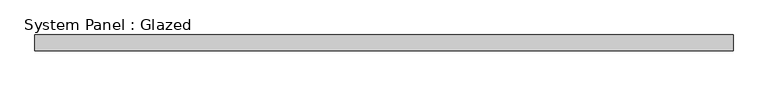
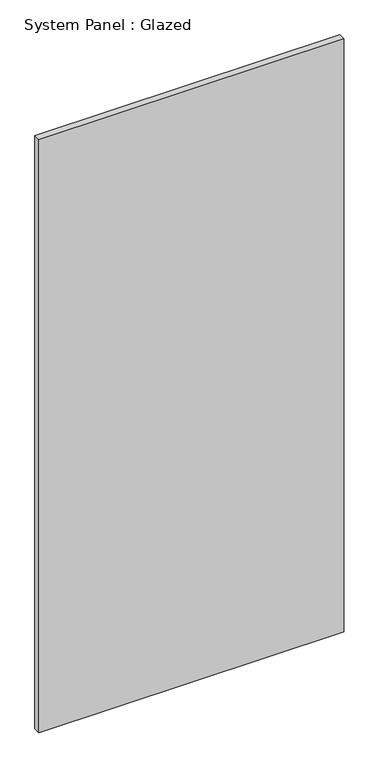
"""IFC4 building model written with IfcOpenShell, lengths in millimetres: plate geometry, System Panel : Glazed."""

from ifc_helpers import new_model, si_unit, origin, origin_with_axes, place, context, project, spatial, polyline, outline, extrude, source, transform, mapped, element, save


def system_panel_glazed_1974f2ce(model_context):
    return source(origin(), model_context, "Body", "SweptSolid", [
        extrude(outline(polyline([(561.975, 19.05), (-561.975, 19.05), (-561.975, 44.45), (561.975, 44.45), (561.975, 19.05)])), origin_with_axes(), (0.0, 0.0, 1.0), 2311.4),
    ])


if __name__ == "__main__":
    model = new_model("IFC4")
    model_context = context("Model", 3, world=origin())
    ifc_project = project(units=[si_unit("LENGTHUNIT", "METRE", prefix="MILLI")], contexts=[model_context])
    site = spatial("IfcSite", under=ifc_project)
    building = spatial("IfcBuilding", under=site)
    placement = place(None, origin())
    system_panel_glazed_shape = system_panel_glazed_1974f2ce(model_context)
    element("IfcPlate", 1, ObjectType="System Panel : Glazed", at=placement, inside=building, context=model_context, shape_type="MappedRepresentation", body=[
        mapped(system_panel_glazed_shape, transform((0.0, 0.0, 0.0), x_axis=(1.0, 0.0, 0.0), y_axis=(0.0, 1.0, 0.0), z_axis=(0.0, 0.0, 1.0))),
    ])
    save(model, "model.ifc")

# Revit data of these elements
# Type "System Panel : Glazed"
#   Construction Type Id = "GSP4R"
#   Analytic Construction = "1/8 in Pilkington single glazing"
#   Visual Light Transmittance = 0.9
#   Solar Heat Gain Coefficient = 0.86
#   Heat Transfer Coefficient (U) = 1.18115 BTU/(h·ft²·°F)
# Element 1 (IfcPlate, "System Panel : Glazed")
#   Materials on its faces: "Glass"
# Materials
#   "Glass": class "Glass", colour RGB 0 128 192, transparency 0.75, Description = "Soda Lime Glass", Cost = 0
